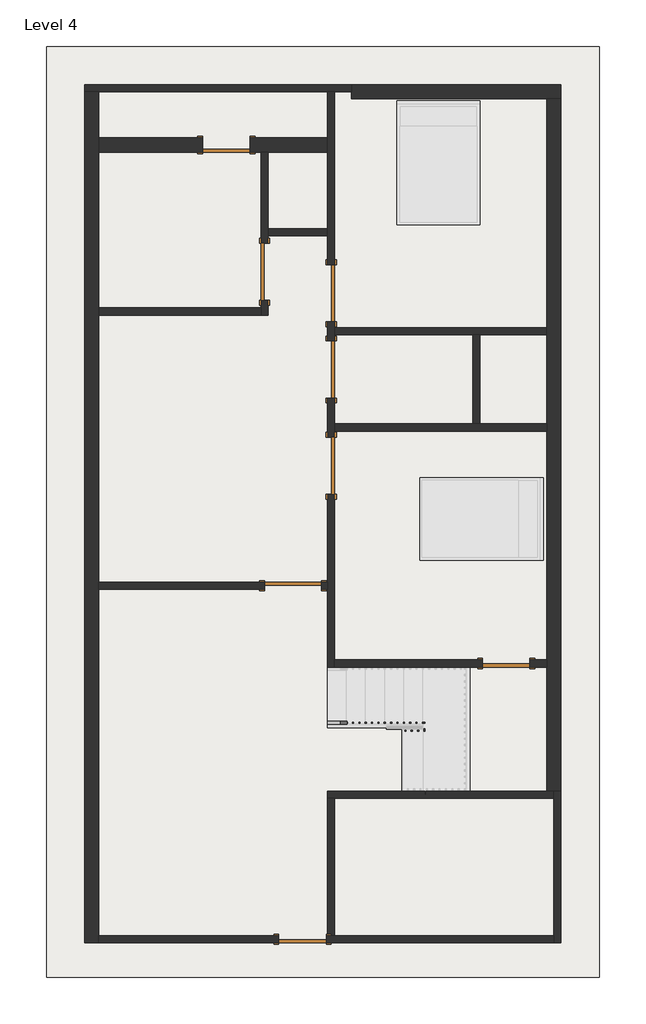
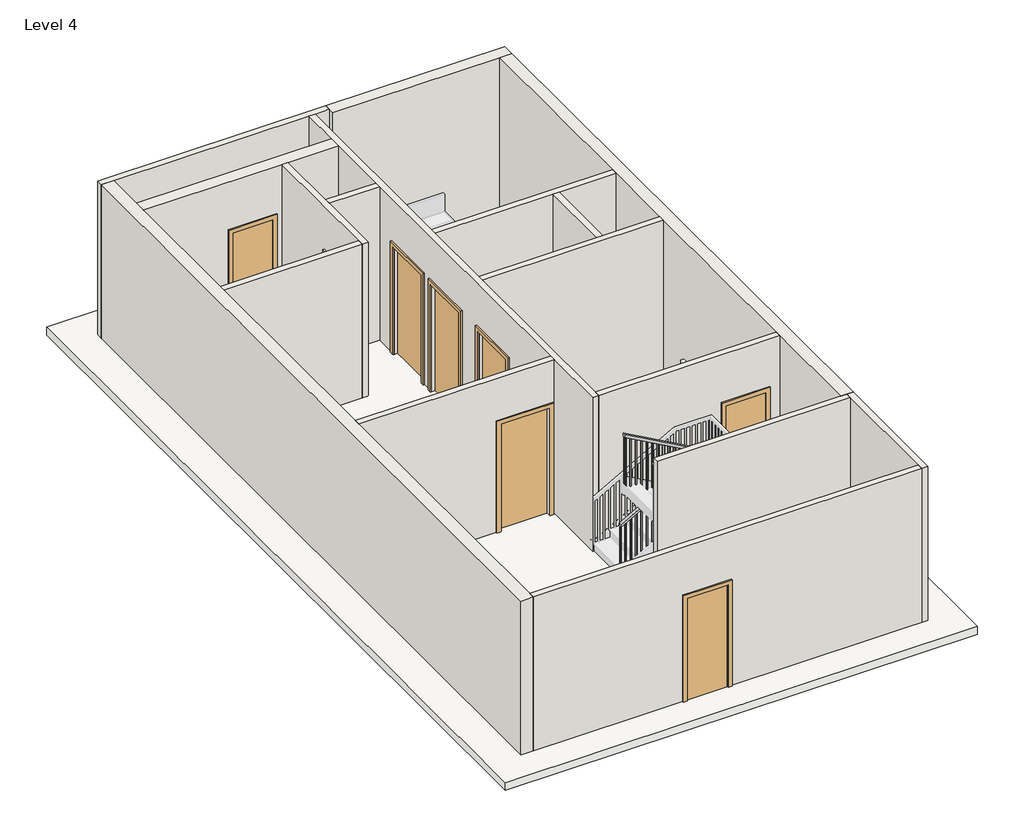
# One storey, part 1 of 2: 18 walls, 8 doors, 1 railing, 1 roof.
"""IFC4 building model written with IfcOpenShell, lengths in millimetres."""

from ifc_helpers import new_model, si_unit, frame, origin, place, context, project, spatial, polyline, outline, extrude, faceted_brep, transform, mapped, element, save
from components import door_85036156, door_d8f5dbb5, door_305aa2a5, door_e5f9f3c4

model = new_model("IFC4")

# Units and contexts
model_context = context("Model", 3, world=origin())
ifc_project = project(units=[si_unit("LENGTHUNIT", "METRE", prefix="MILLI")], contexts=[model_context])

# Site, building, storey
site = spatial("IfcSite", under=ifc_project)
building = spatial("IfcBuilding", under=site)
storey = spatial("IfcBuildingStorey", under=building, Name="Level 4", Elevation=6400.8)

# Doors
placement = place(None, origin())
door_shape = door_85036156(model_context)
element("IfcDoor", 1, ObjectType="Single-Flush : 30\" x 80\"", at=placement, inside=storey, context=model_context, shape_type="MappedRepresentation", body=[
    mapped(door_shape, transform((-2798.2915084, 6430.9935985, 6400.8), x_axis=(1.0, 0.0, 0.0), y_axis=(0.0, 1.0, 0.0), z_axis=(0.0, 0.0, 1.0))),
])
door_2_shape = door_d8f5dbb5(model_context)
element("IfcDoor", 2, ObjectType="Single-Flush : 30\" x 80\"", at=placement, inside=storey, context=model_context, shape_type="MappedRepresentation", body=[
    mapped(door_2_shape, transform((1678.4584916, -1855.7564015, 6400.8), x_axis=(-1.0, 0.0, 0.0), y_axis=(0.0, -1.0, 0.0), z_axis=(0.0, 0.0, 1.0))),
])
element("IfcDoor", 3, ObjectType="Single-Flush : 30\" x 80\"", at=placement, inside=storey, context=model_context, shape_type="MappedRepresentation", body=[
    mapped(door_2_shape, transform((-1579.0915084, -6262.6564015, 6400.8), x_axis=(-1.0, 0.0, 0.0), y_axis=(0.0, -1.0, 0.0), z_axis=(0.0, 0.0, 1.0))),
])
door_3_shape = door_305aa2a5(model_context)
element("IfcDoor", 4, ObjectType="Single-Flush : 36\" x 84\"", at=placement, inside=storey, context=model_context, shape_type="MappedRepresentation", body=[
    mapped(door_3_shape, transform((-2188.6915084, 4405.3435985, 6400.8), x_axis=(0.0, -1.0, 0.0), y_axis=(1.0, 0.0, 0.0), z_axis=(0.0, 0.0, 1.0))),
])
element("IfcDoor", 5, ObjectType="Single-Flush : 36\" x 84\"", at=placement, inside=storey, context=model_context, shape_type="MappedRepresentation", body=[
    mapped(door_3_shape, transform((-1121.8915084, 1306.5435985, 6400.8), x_axis=(0.0, 1.0, 0.0), y_axis=(-1.0, 0.0, 0.0), z_axis=(0.0, 0.0, 1.0))),
])
door_4_shape = door_e5f9f3c4(model_context)
element("IfcDoor", 6, ObjectType="Single-Flush : 36\" x 84\"", at=placement, inside=storey, context=model_context, shape_type="MappedRepresentation", body=[
    mapped(door_4_shape, transform((-1121.8915084, 4062.4435985, 6400.8), x_axis=(0.0, -1.0, 0.0), y_axis=(1.0, 0.0, 0.0), z_axis=(0.0, 0.0, 1.0))),
])
element("IfcDoor", 7, ObjectType="Single-Flush : 36\" x 84\"", at=placement, inside=storey, context=model_context, shape_type="MappedRepresentation", body=[
    mapped(door_4_shape, transform((-1121.8915084, 2843.2435985, 6400.8), x_axis=(0.0, -1.0, 0.0), y_axis=(1.0, 0.0, 0.0), z_axis=(0.0, 0.0, 1.0))),
])
element("IfcDoor", 8, ObjectType="Single-Flush : 36\" x 84\"", at=placement, inside=storey, context=model_context, shape_type="MappedRepresentation", body=[
    mapped(door_4_shape, transform((-1731.4915084, -611.1564015, 6400.8), x_axis=(1.0, 0.0, 0.0), y_axis=(0.0, 1.0, 0.0), z_axis=(0.0, 0.0, 1.0))),
])

# Railing
element("IfcRailing", 9, ObjectType="Handrail - Rectangular", at=placement, inside=storey, context=model_context, shape_type="SolidModel", body=[
    faceted_brep([(-1179.0415084, -2776.5064015, 7484.5333333), (-1179.0415084, -2776.5064015, 7426.420221), (-1179.0415084, -2827.3064015, 7426.420221), (-1179.0415084, -2827.3064015, 7484.5333333), (268.7584916, -2776.5064015, 8288.8666667), (319.5584916, -2776.5064015, 8258.9757765), (319.5584916, -2827.3064015, 8258.9757765), (268.7584916, -2827.3064015, 8288.8666667), (268.7584916, -2776.5064015, 8331.2), (319.5584916, -2776.5064015, 8280.4), (319.5584916, -2827.3064015, 8280.4), (268.7584916, -2827.3064015, 8331.2), (395.7584916, -2776.5064015, 8331.2), (395.7584916, -2776.5064015, 8280.4), (344.9584916, -2827.3064015, 8280.4), (344.9584916, -2827.3064015, 8331.2), (395.7584916, -2903.5064015, 8331.2), (395.7584916, -2903.5064015, 8280.4), (344.9584916, -2903.5064015, 8280.4), (344.9584916, -2903.5064015, 8331.2), (395.7584916, -2928.9064015, 8331.2), (344.9584916, -2928.9064015, 8331.2), (344.9584916, -2928.9064015, 8280.4), (395.7584916, -2928.9064015, 8280.4)], [[[0, 1, 2, 3]], [[1, 0, 4, 5]], [[2, 1, 5, 6]], [[3, 2, 6, 7]], [[0, 3, 7, 4]], [[5, 4, 8, 9]], [[6, 5, 9, 10]], [[7, 6, 10, 11]], [[4, 7, 11, 8]], [[9, 8, 12, 13]], [[10, 9, 13, 14]], [[11, 10, 14, 15]], [[8, 11, 15, 12]], [[13, 12, 16, 17]], [[14, 13, 17, 18]], [[15, 14, 18, 19]], [[12, 15, 19, 16]], [[20, 21, 22, 23]], [[17, 16, 20, 23]], [[18, 17, 23, 22]], [[19, 18, 22, 21]], [[16, 19, 21, 20]]]),
    faceted_brep([(395.7584916, -2903.5064015, 8331.2), (395.7584916, -2954.3064015, 8280.4), (344.9584916, -2954.3064015, 8280.4), (344.9584916, -2903.5064015, 8331.2), (395.7584916, -2903.5064015, 8472.3111111), (344.9584916, -2903.5064015, 8442.420221), (344.9584916, -2954.3064015, 8442.420221), (395.7584916, -2954.3064015, 8472.3111111)], [[[0, 1, 2, 3]], [[4, 5, 6, 7]], [[1, 0, 4, 7]], [[2, 1, 7, 6]], [[3, 2, 6, 5]], [[0, 3, 5, 4]]]),
    faceted_brep([(395.7584916, -2954.3064015, 8472.3111111), (344.9584916, -2954.3064015, 8442.420221), (344.9584916, -2903.5064015, 8442.420221), (395.7584916, -2903.5064015, 8472.3111111), (-1179.0415084, -2954.3064015, 9347.2), (-1179.0415084, -2903.5064015, 9347.2), (-1179.0415084, -2903.5064015, 9289.0868876), (-1179.0415084, -2954.3064015, 9289.0868876)], [[[0, 1, 2, 3]], [[4, 5, 6, 7]], [[1, 0, 4, 7]], [[2, 1, 7, 6]], [[3, 2, 6, 5]], [[0, 3, 5, 4]]]),
    extrude(outline(polyline([(9269.6841099, -1144.1165084), (9280.2674432, -1163.1665084), (8263.4666667, -1163.1665084), (8263.4666667, -1144.1165084), (9269.6841099, -1144.1165084)])), frame((0.0, -2938.4314015, 0.0), z_axis=(0.0, 1.0, 0.0), x_axis=(0.0, 0.0, 1.0)), (0.0, 0.0, 1.0), 19.05),
    extrude(outline(polyline([(9213.2396654, -1042.5165084), (9223.8229988, -1061.5665084), (8263.4666667, -1061.5665084), (8263.4666667, -1042.5165084), (9213.2396654, -1042.5165084)])), frame((0.0, -2938.4314015, 0.0), z_axis=(0.0, 1.0, 0.0), x_axis=(0.0, 0.0, 1.0)), (0.0, 0.0, 1.0), 19.05),
    extrude(outline(polyline([(9156.795221, -940.9165084), (9167.3785543, -959.9665084), (8263.4666667, -959.9665084), (8263.4666667, -940.9165084), (9156.795221, -940.9165084)])), frame((0.0, -2938.4314015, 0.0), z_axis=(0.0, 1.0, 0.0), x_axis=(0.0, 0.0, 1.0)), (0.0, 0.0, 1.0), 19.05),
    extrude(outline(polyline([(9100.3507765, -839.3165084), (9110.9341099, -858.3665084), (8094.1333333, -858.3665084), (8094.1333333, -839.3165084), (9100.3507765, -839.3165084)])), frame((0.0, -2938.4314015, 0.0), z_axis=(0.0, 1.0, 0.0), x_axis=(0.0, 0.0, 1.0)), (0.0, 0.0, 1.0), 19.05),
    extrude(outline(polyline([(9043.9063321, -737.7165084), (9054.4896654, -756.7665084), (8094.1333333, -756.7665084), (8094.1333333, -737.7165084), (9043.9063321, -737.7165084)])), frame((0.0, -2938.4314015, 0.0), z_axis=(0.0, 1.0, 0.0), x_axis=(0.0, 0.0, 1.0)), (0.0, 0.0, 1.0), 19.05),
    extrude(outline(polyline([(8987.4618876, -636.1165084), (8998.045221, -655.1665084), (8094.1333333, -655.1665084), (8094.1333333, -636.1165084), (8987.4618876, -636.1165084)])), frame((0.0, -2938.4314015, 0.0), z_axis=(0.0, 1.0, 0.0), x_axis=(0.0, 0.0, 1.0)), (0.0, 0.0, 1.0), 19.05),
    extrude(outline(polyline([(8931.0174432, -534.5165084), (8941.6007765, -553.5665084), (7924.8, -553.5665084), (7924.8, -534.5165084), (8931.0174432, -534.5165084)])), frame((0.0, -2938.4314015, 0.0), z_axis=(0.0, 1.0, 0.0), x_axis=(0.0, 0.0, 1.0)), (0.0, 0.0, 1.0), 19.05),
    extrude(outline(polyline([(8874.5729988, -432.9165084), (8885.1563321, -451.9665084), (7924.8, -451.9665084), (7924.8, -432.9165084), (8874.5729988, -432.9165084)])), frame((0.0, -2938.4314015, 0.0), z_axis=(0.0, 1.0, 0.0), x_axis=(0.0, 0.0, 1.0)), (0.0, 0.0, 1.0), 19.05),
    extrude(outline(polyline([(8818.1285543, -331.3165084), (8828.7118876, -350.3665084), (7924.8, -350.3665084), (7924.8, -331.3165084), (8818.1285543, -331.3165084)])), frame((0.0, -2938.4314015, 0.0), z_axis=(0.0, 1.0, 0.0), x_axis=(0.0, 0.0, 1.0)), (0.0, 0.0, 1.0), 19.05),
    extrude(outline(polyline([(8761.6841099, -229.7165084), (8772.2674432, -248.7665084), (7755.4666667, -248.7665084), (7755.4666667, -229.7165084), (8761.6841099, -229.7165084)])), frame((0.0, -2938.4314015, 0.0), z_axis=(0.0, 1.0, 0.0), x_axis=(0.0, 0.0, 1.0)), (0.0, 0.0, 1.0), 19.05),
    extrude(outline(polyline([(8705.2396654, -128.1165084), (8715.8229988, -147.1665084), (7755.4666667, -147.1665084), (7755.4666667, -128.1165084), (8705.2396654, -128.1165084)])), frame((0.0, -2938.4314015, 0.0), z_axis=(0.0, 1.0, 0.0), x_axis=(0.0, 0.0, 1.0)), (0.0, 0.0, 1.0), 19.05),
    extrude(outline(polyline([(8648.795221, -26.5165084), (8659.3785543, -45.5665084), (7755.4666667, -45.5665084), (7755.4666667, -26.5165084), (8648.795221, -26.5165084)])), frame((0.0, -2938.4314015, 0.0), z_axis=(0.0, 1.0, 0.0), x_axis=(0.0, 0.0, 1.0)), (0.0, 0.0, 1.0), 19.05),
    extrude(outline(polyline([(8592.3507765, 75.0834916), (8602.9341099, 56.0334916), (7586.1333333, 56.0334916), (7586.1333333, 75.0834916), (8592.3507765, 75.0834916)])), frame((0.0, -2938.4314015, 0.0), z_axis=(0.0, 1.0, 0.0), x_axis=(0.0, 0.0, 1.0)), (0.0, 0.0, 1.0), 19.05),
    extrude(outline(polyline([(8535.9063321, 176.6834916), (8546.4896654, 157.6334916), (7586.1333333, 157.6334916), (7586.1333333, 176.6834916), (8535.9063321, 176.6834916)])), frame((0.0, -2938.4314015, 0.0), z_axis=(0.0, 1.0, 0.0), x_axis=(0.0, 0.0, 1.0)), (0.0, 0.0, 1.0), 19.05),
    extrude(outline(polyline([(8479.4618876, 278.2834916), (8490.045221, 259.2334916), (7586.1333333, 259.2334916), (7586.1333333, 278.2834916), (8479.4618876, 278.2834916)])), frame((0.0, -2938.4314015, 0.0), z_axis=(0.0, 1.0, 0.0), x_axis=(0.0, 0.0, 1.0)), (0.0, 0.0, 1.0), 19.05),
    extrude(outline(polyline([(360.8334916, -2893.9814015), (379.8834916, -2893.9814015), (379.8834916, -2913.0314015), (360.8334916, -2913.0314015), (360.8334916, -2893.9814015)])), frame((0.0, 0.0, 7416.8), z_axis=(0.0, 0.0, 1.0), x_axis=(1.0, 0.0, 0.0)), (0.0, 0.0, 1.0), 863.6),
    extrude(outline(polyline([(335.4334916, -2811.4314015), (335.4334916, -2792.3814015), (354.4834916, -2792.3814015), (354.4834916, -2811.4314015), (335.4334916, -2811.4314015)])), frame((0.0, 0.0, 7416.8), z_axis=(0.0, 0.0, 1.0), x_axis=(1.0, 0.0, 0.0)), (0.0, 0.0, 1.0), 863.6),
    extrude(outline(polyline([(8221.9341099, 252.8834916), (8211.3507765, 233.8334916), (7247.4666667, 233.8334916), (7247.4666667, 252.8834916), (8221.9341099, 252.8834916)])), frame((0.0, -2811.4314015, 0.0), z_axis=(0.0, 1.0, 0.0), x_axis=(0.0, 0.0, 1.0)), (0.0, 0.0, 1.0), 19.05),
    extrude(outline(polyline([(8165.4896654, 151.2834916), (8154.9063321, 132.2334916), (7247.4666667, 132.2334916), (7247.4666667, 151.2834916), (8165.4896654, 151.2834916)])), frame((0.0, -2811.4314015, 0.0), z_axis=(0.0, 1.0, 0.0), x_axis=(0.0, 0.0, 1.0)), (0.0, 0.0, 1.0), 19.05),
    extrude(outline(polyline([(8109.045221, 49.6834916), (8098.4618876, 30.6334916), (7247.4666667, 30.6334916), (7247.4666667, 49.6834916), (8109.045221, 49.6834916)])), frame((0.0, -2811.4314015, 0.0), z_axis=(0.0, 1.0, 0.0), x_axis=(0.0, 0.0, 1.0)), (0.0, 0.0, 1.0), 19.05),
    extrude(outline(polyline([(8052.6007765, -51.9165084), (8042.0174432, -70.9665084), (7078.1333333, -70.9665084), (7078.1333333, -51.9165084), (8052.6007765, -51.9165084)])), frame((0.0, -2811.4314015, 0.0), z_axis=(0.0, 1.0, 0.0), x_axis=(0.0, 0.0, 1.0)), (0.0, 0.0, 1.0), 19.05),
    extrude(outline(polyline([(7996.1563321, -153.5165084), (7985.5729988, -172.5665084), (7078.1333333, -172.5665084), (7078.1333333, -153.5165084), (7996.1563321, -153.5165084)])), frame((0.0, -2811.4314015, 0.0), z_axis=(0.0, 1.0, 0.0), x_axis=(0.0, 0.0, 1.0)), (0.0, 0.0, 1.0), 19.05),
    extrude(outline(polyline([(7939.7118876, -255.1165084), (7929.1285543, -274.1665084), (7078.1333333, -274.1665084), (7078.1333333, -255.1165084), (7939.7118876, -255.1165084)])), frame((0.0, -2811.4314015, 0.0), z_axis=(0.0, 1.0, 0.0), x_axis=(0.0, 0.0, 1.0)), (0.0, 0.0, 1.0), 19.05),
    extrude(outline(polyline([(7883.2674432, -356.7165084), (7872.6841099, -375.7665084), (6908.8, -375.7665084), (6908.8, -356.7165084), (7883.2674432, -356.7165084)])), frame((0.0, -2811.4314015, 0.0), z_axis=(0.0, 1.0, 0.0), x_axis=(0.0, 0.0, 1.0)), (0.0, 0.0, 1.0), 19.05),
    extrude(outline(polyline([(7826.8229988, -458.3165084), (7816.2396654, -477.3665084), (6908.8, -477.3665084), (6908.8, -458.3165084), (7826.8229988, -458.3165084)])), frame((0.0, -2811.4314015, 0.0), z_axis=(0.0, 1.0, 0.0), x_axis=(0.0, 0.0, 1.0)), (0.0, 0.0, 1.0), 19.05),
    extrude(outline(polyline([(7770.3785543, -559.9165084), (7759.795221, -578.9665084), (6908.8, -578.9665084), (6908.8, -559.9165084), (7770.3785543, -559.9165084)])), frame((0.0, -2811.4314015, 0.0), z_axis=(0.0, 1.0, 0.0), x_axis=(0.0, 0.0, 1.0)), (0.0, 0.0, 1.0), 19.05),
    extrude(outline(polyline([(7713.9341099, -661.5165084), (7703.3507765, -680.5665084), (6739.4666667, -680.5665084), (6739.4666667, -661.5165084), (7713.9341099, -661.5165084)])), frame((0.0, -2811.4314015, 0.0), z_axis=(0.0, 1.0, 0.0), x_axis=(0.0, 0.0, 1.0)), (0.0, 0.0, 1.0), 19.05),
    extrude(outline(polyline([(7657.4896654, -763.1165084), (7646.9063321, -782.1665084), (6739.4666667, -782.1665084), (6739.4666667, -763.1165084), (7657.4896654, -763.1165084)])), frame((0.0, -2811.4314015, 0.0), z_axis=(0.0, 1.0, 0.0), x_axis=(0.0, 0.0, 1.0)), (0.0, 0.0, 1.0), 19.05),
    extrude(outline(polyline([(7601.045221, -864.7165084), (7590.4618876, -883.7665084), (6739.4666667, -883.7665084), (6739.4666667, -864.7165084), (7601.045221, -864.7165084)])), frame((0.0, -2811.4314015, 0.0), z_axis=(0.0, 1.0, 0.0), x_axis=(0.0, 0.0, 1.0)), (0.0, 0.0, 1.0), 19.05),
    extrude(outline(polyline([(7544.6007765, -966.3165084), (7534.0174432, -985.3665084), (6570.1333333, -985.3665084), (6570.1333333, -966.3165084), (7544.6007765, -966.3165084)])), frame((0.0, -2811.4314015, 0.0), z_axis=(0.0, 1.0, 0.0), x_axis=(0.0, 0.0, 1.0)), (0.0, 0.0, 1.0), 19.05),
    extrude(outline(polyline([(7488.1563321, -1067.9165084), (7477.5729988, -1086.9665084), (6570.1333333, -1086.9665084), (6570.1333333, -1067.9165084), (7488.1563321, -1067.9165084)])), frame((0.0, -2811.4314015, 0.0), z_axis=(0.0, 1.0, 0.0), x_axis=(0.0, 0.0, 1.0)), (0.0, 0.0, 1.0), 19.05),
    extrude(outline(polyline([(360.8334916, -2919.3814015), (379.8834916, -2919.3814015), (379.8834916, -2938.4314015), (360.8334916, -2938.4314015), (360.8334916, -2919.3814015)])), frame((0.0, 0.0, 7416.8), z_axis=(0.0, 0.0, 1.0), x_axis=(1.0, 0.0, 0.0)), (0.0, 0.0, 1.0), 863.6),
    extrude(outline(polyline([(360.8334916, -2811.4314015), (360.8334916, -2792.3814015), (379.8834916, -2792.3814015), (379.8834916, -2811.4314015), (360.8334916, -2811.4314015)])), frame((0.0, 0.0, 7416.8), z_axis=(0.0, 0.0, 1.0), x_axis=(1.0, 0.0, 0.0)), (0.0, 0.0, 1.0), 863.6),
    extrude(outline(polyline([(9278.5035543, -1159.9915084), (9289.0868876, -1179.0415084), (8263.4666667, -1179.0415084), (8263.4666667, -1159.9915084), (9278.5035543, -1159.9915084)])), frame((0.0, -2938.4314015, 0.0), z_axis=(0.0, 1.0, 0.0), x_axis=(0.0, 0.0, 1.0)), (0.0, 0.0, 1.0), 19.05),
    extrude(outline(polyline([(7437.0035543, -1159.9915084), (7426.420221, -1179.0415084), (6570.1333333, -1179.0415084), (6570.1333333, -1159.9915084), (7437.0035543, -1159.9915084)])), frame((0.0, -2811.4314015, 0.0), z_axis=(0.0, 1.0, 0.0), x_axis=(0.0, 0.0, 1.0)), (0.0, 0.0, 1.0), 19.05),
])

# Roof
element("IfcRoof", 10, ObjectType="Generic - 12\"", at=placement, inside=storey, context=model_context, shape_type="SweptSolid", body=[
    extrude(outline(polyline([(-5674.8415084, 8005.7935985), (3164.3584916, 8005.7935985), (3164.3584916, -6872.2564015), (-5674.8415084, -6872.2564015), (-5674.8415084, 8005.7935985)])), frame((0.0, 0.0, 6248.4), z_axis=(0.0, 0.0, 1.0), x_axis=(1.0, 0.0, 0.0)), (0.0, 0.0, 1.0), 152.4),
])

# Walls
element("IfcWall", 11, ObjectType="WALL 9\"", at=placement, inside=storey, context=model_context, shape_type="Brep", body=[
    faceted_brep([(-798.0415084, 7167.5935985, 6400.8), (2326.1584916, 7167.5935985, 6400.8), (2554.7584916, 7167.5935985, 6400.8), (2554.7584916, 7167.5935985, 9448.8), (2326.1584916, 7167.5935985, 9448.8), (-798.0415084, 7167.5935985, 9448.8), (-798.0415084, 7396.1935985, 6400.8), (-798.0415084, 7396.1935985, 9448.8), (2554.7584916, 7396.1935985, 9448.8), (2554.7584916, 7396.1935985, 6400.8), (-798.0415084, 7281.8935985, 6400.8), (-798.0415084, 7281.8935985, 9448.8)], [[[0, 1, 2, 3, 4, 5]], [[6, 7, 8, 9]], [[2, 1, 0, 10, 6, 9]], [[5, 4, 3, 8, 7, 11]], [[0, 5, 11, 7, 6, 10]], [[3, 2, 9, 8]]]),
])
element("IfcWall", 12, ObjectType="WALL 9\"", at=placement, inside=storey, context=model_context, shape_type="Brep", body=[
    faceted_brep([(2326.1584916, 7167.5935985, 6400.8), (2326.1584916, 3509.9935985, 6400.8), (2326.1584916, 3395.6935985, 6400.8), (2326.1584916, 1973.2935985, 6400.8), (2326.1584916, 1858.9935985, 6400.8), (2326.1584916, -1798.6064015, 6400.8), (2326.1584916, -1912.9064015, 6400.8), (2326.1584916, -3894.1064015, 6400.8), (2326.1584916, -3894.1064015, 9448.8), (2326.1584916, -1912.9064015, 9448.8), (2326.1584916, -1798.6064015, 9448.8), (2326.1584916, 1858.9935985, 9448.8), (2326.1584916, 1973.2935985, 9448.8), (2326.1584916, 3395.6935985, 9448.8), (2326.1584916, 3509.9935985, 9448.8), (2326.1584916, 7167.5935985, 9448.8), (2554.7584916, 7167.5935985, 6400.8), (2554.7584916, 7167.5935985, 9448.8), (2554.7584916, -3894.1064015, 9448.8), (2554.7584916, -3894.1064015, 6400.8), (2440.4584916, -3894.1064015, 6400.8), (2440.4584916, -3894.1064015, 9448.8)], [[[0, 1, 2, 3, 4, 5, 6, 7, 8, 9, 10, 11, 12, 13, 14, 15]], [[16, 17, 18, 19]], [[7, 6, 5, 4, 3, 2, 1, 0, 16, 19, 20]], [[15, 14, 13, 12, 11, 10, 9, 8, 21, 18, 17]], [[0, 15, 17, 16]], [[8, 7, 20, 19, 18, 21]]]),
])
element("IfcWall", 13, ObjectType="WALL 9\"", at=placement, inside=storey, context=model_context, shape_type="Brep", body=[
    faceted_brep([(-5065.2415084, 7281.8935985, 6400.8), (-5065.2415084, -6319.8064015, 6400.8), (-5065.2415084, -6319.8064015, 9448.8), (-5065.2415084, 7281.8935985, 9448.8), (-4836.6415084, 7281.8935985, 6400.8), (-4836.6415084, 7281.8935985, 9448.8), (-4836.6415084, 6545.2935985, 9448.8), (-4836.6415084, 6316.6935985, 9448.8), (-4836.6415084, 3827.4935985, 9448.8), (-4836.6415084, 3713.1935985, 9448.8), (-4836.6415084, -554.0064015, 9448.8), (-4836.6415084, -668.3064015, 9448.8), (-4836.6415084, -6205.5064015, 9448.8), (-4836.6415084, -6319.8064015, 9448.8), (-4836.6415084, -6319.8064015, 6400.8), (-4836.6415084, -6205.5064015, 6400.8), (-4836.6415084, -668.3064015, 6400.8), (-4836.6415084, -554.0064015, 6400.8), (-4836.6415084, 3713.1935985, 6400.8), (-4836.6415084, 3827.4935985, 6400.8), (-4836.6415084, 6316.6935985, 6400.8), (-4836.6415084, 6545.2935985, 6400.8)], [[[0, 1, 2, 3]], [[4, 5, 6, 7, 8, 9, 10, 11, 12, 13, 14, 15, 16, 17, 18, 19, 20, 21]], [[1, 0, 4, 21, 20, 19, 18, 17, 16, 15, 14]], [[3, 2, 13, 12, 11, 10, 9, 8, 7, 6, 5]], [[0, 3, 5, 4]], [[2, 1, 14, 13]]]),
])
element("IfcWall", 14, ObjectType="WALL 9\"", at=placement, inside=storey, context=model_context, shape_type="Brep", body=[
    faceted_brep([(-2417.2915084, 6316.6935985, 8432.8), (-2417.2915084, 6316.6935985, 6400.8), (-2245.8415084, 6316.6935985, 6400.8), (-2131.5415084, 6316.6935985, 6400.8), (-1179.0415084, 6316.6935985, 6400.8), (-1179.0415084, 6316.6935985, 9448.8), (-2131.5415084, 6316.6935985, 9448.8), (-2245.8415084, 6316.6935985, 9448.8), (-4836.6415084, 6316.6935985, 9448.8), (-4836.6415084, 6316.6935985, 6400.8), (-3179.2915084, 6316.6935985, 6400.8), (-3179.2915084, 6316.6935985, 8432.8), (-1179.0415084, 6545.2935985, 6400.8), (-2417.2915084, 6545.2935985, 6400.8), (-2417.2915084, 6545.2935985, 8432.8), (-3179.2915084, 6545.2935985, 8432.8), (-3179.2915084, 6545.2935985, 6400.8), (-4836.6415084, 6545.2935985, 6400.8), (-4836.6415084, 6545.2935985, 9448.8), (-1179.0415084, 6545.2935985, 9448.8)], [[[0, 1, 2, 3, 4, 5, 6, 7, 8, 9, 10, 11]], [[12, 13, 14, 15, 16, 17, 18, 19]], [[10, 9, 17, 16]], [[4, 3, 2, 1, 13, 12]], [[8, 7, 6, 5, 19, 18]], [[9, 8, 18, 17]], [[5, 4, 12, 19]], [[14, 13, 1, 0]], [[15, 14, 0, 11]], [[16, 15, 11, 10]]]),
])
element("IfcWall", 15, ObjectType="WALL4.5\"", at=placement, inside=storey, context=model_context, shape_type="Brep", body=[
    faceted_brep([(-5065.2415084, 7281.8935985, 6400.8), (-4836.6415084, 7281.8935985, 6400.8), (-1179.0415084, 7281.8935985, 6400.8), (-1064.7415084, 7281.8935985, 6400.8), (-798.0415084, 7281.8935985, 6400.8), (-798.0415084, 7281.8935985, 9448.8), (-1064.7415084, 7281.8935985, 9448.8), (-1179.0415084, 7281.8935985, 9448.8), (-4836.6415084, 7281.8935985, 9448.8), (-5065.2415084, 7281.8935985, 9448.8), (-5065.2415084, 7396.1935985, 6400.8), (-5065.2415084, 7396.1935985, 9448.8), (-798.0415084, 7396.1935985, 9448.8), (-798.0415084, 7396.1935985, 6400.8)], [[[0, 1, 2, 3, 4, 5, 6, 7, 8, 9]], [[10, 11, 12, 13]], [[4, 3, 2, 1, 0, 10, 13]], [[5, 4, 13, 12]], [[9, 8, 7, 6, 5, 12, 11]], [[0, 9, 11, 10]]]),
])
element("IfcWall", 16, ObjectType="WALL4.5\"", at=placement, inside=storey, context=model_context, shape_type="Brep", body=[
    faceted_brep([(2554.7584916, -6319.8064015, 6400.8), (2554.7584916, -3894.1064015, 6400.8), (2554.7584916, -3894.1064015, 9448.8), (2554.7584916, -6319.8064015, 9448.8), (2440.4584916, -6319.8064015, 6400.8), (2440.4584916, -6319.8064015, 9448.8), (2440.4584916, -6205.5064015, 9448.8), (2440.4584916, -4008.4064015, 9448.8), (2440.4584916, -3894.1064015, 9448.8), (2440.4584916, -3894.1064015, 6400.8), (2440.4584916, -4008.4064015, 6400.8), (2440.4584916, -6205.5064015, 6400.8)], [[[0, 1, 2, 3]], [[4, 5, 6, 7, 8, 9, 10, 11]], [[1, 0, 4, 11, 10, 9]], [[3, 2, 8, 7, 6, 5]], [[2, 1, 9, 8]], [[0, 3, 5, 4]]]),
])
element("IfcWall", 17, ObjectType="WALL4.5\"", at=placement, inside=storey, context=model_context, shape_type="Brep", body=[
    faceted_brep([(2440.4584916, -3894.1064015, 6400.8), (2326.1584916, -3894.1064015, 6400.8), (-1179.0415084, -3894.1064015, 6400.8), (-1179.0415084, -3894.1064015, 9448.8), (2326.1584916, -3894.1064015, 9448.8), (2440.4584916, -3894.1064015, 9448.8), (2440.4584916, -4008.4064015, 6400.8), (2440.4584916, -4008.4064015, 9448.8), (-1179.0415084, -4008.4064015, 9448.8), (-1179.0415084, -4008.4064015, 7620.0), (-1179.0415084, -4008.4064015, 6400.8), (-1064.7415084, -4008.4064015, 6400.8)], [[[0, 1, 2, 3, 4, 5]], [[6, 7, 8, 9, 10, 11]], [[2, 1, 0, 6, 11, 10]], [[5, 4, 3, 8, 7]], [[0, 5, 7, 6]], [[3, 2, 10, 9, 8]]]),
])
element("IfcWall", 18, ObjectType="WALL4.5\"", at=placement, inside=storey, context=model_context, shape_type="Brep", body=[
    faceted_brep([(-2245.8415084, 3948.1435985, 8534.4), (-2245.8415084, 3948.1435985, 6400.8), (-2245.8415084, 3827.4935985, 6400.8), (-2245.8415084, 3713.1935985, 6400.8), (-2245.8415084, 3713.1935985, 9448.8), (-2245.8415084, 3827.4935985, 9448.8), (-2245.8415084, 6316.6935985, 9448.8), (-2245.8415084, 6316.6935985, 6400.8), (-2245.8415084, 4862.5435985, 6400.8), (-2245.8415084, 4862.5435985, 8534.4), (-2131.5415084, 3713.1935985, 6400.8), (-2131.5415084, 3948.1435985, 6400.8), (-2131.5415084, 3948.1435985, 8534.4), (-2131.5415084, 4862.5435985, 8534.4), (-2131.5415084, 4862.5435985, 6400.8), (-2131.5415084, 4983.1935985, 6400.8), (-2131.5415084, 5097.4935985, 6400.8), (-2131.5415084, 6316.6935985, 6400.8), (-2131.5415084, 6316.6935985, 9448.8), (-2131.5415084, 5097.4935985, 9448.8), (-2131.5415084, 4983.1935985, 9448.8), (-2131.5415084, 3713.1935985, 9448.8)], [[[0, 1, 2, 3, 4, 5, 6, 7, 8, 9]], [[10, 11, 12, 13, 14, 15, 16, 17, 18, 19, 20, 21]], [[8, 7, 17, 16, 15, 14]], [[3, 2, 1, 11, 10]], [[6, 5, 4, 21, 20, 19, 18]], [[7, 6, 18, 17]], [[4, 3, 10, 21]], [[12, 11, 1, 0]], [[13, 12, 0, 9]], [[14, 13, 9, 8]]]),
])
element("IfcWall", 19, ObjectType="WALL4.5\"", at=placement, inside=storey, context=model_context, shape_type="SweptSolid", body=[
    extrude(outline(polyline([(-2245.8415084, 3713.1935985), (-4836.6415084, 3713.1935985), (-4836.6415084, 3827.4935985), (-2245.8415084, 3827.4935985), (-2245.8415084, 3713.1935985)])), frame((0.0, 0.0, 6400.8), z_axis=(0.0, 0.0, 1.0), x_axis=(1.0, 0.0, 0.0)), (0.0, 0.0, 1.0), 3048.0),
])
element("IfcWall", 20, ObjectType="WALL4.5\"", at=placement, inside=storey, context=model_context, shape_type="SweptSolid", body=[
    extrude(outline(polyline([(-1179.0415084, 4983.1935985), (-2131.5415084, 4983.1935985), (-2131.5415084, 5097.4935985), (-1179.0415084, 5097.4935985), (-1179.0415084, 4983.1935985)])), frame((0.0, 0.0, 6400.8), z_axis=(0.0, 0.0, 1.0), x_axis=(1.0, 0.0, 0.0)), (0.0, 0.0, 1.0), 3048.0),
])
element("IfcWall", 21, ObjectType="WALL4.5\"", at=placement, inside=storey, context=model_context, shape_type="Brep", body=[
    faceted_brep([(-1179.0415084, 2386.0435985, 6400.8), (-1179.0415084, 1763.7435985, 6400.8), (-1179.0415084, 1763.7435985, 8534.4), (-1179.0415084, 849.3435985, 8534.4), (-1179.0415084, 849.3435985, 6400.8), (-1179.0415084, -554.0064015, 6400.8), (-1179.0415084, -668.3064015, 6400.8), (-1179.0415084, -1912.9064015, 6400.8), (-1179.0415084, -1912.9064015, 9448.8), (-1179.0415084, -668.3064015, 9448.8), (-1179.0415084, -554.0064015, 9448.8), (-1179.0415084, 4983.1935985, 9448.8), (-1179.0415084, 5097.4935985, 9448.8), (-1179.0415084, 6316.6935985, 9448.8), (-1179.0415084, 6545.2935985, 9448.8), (-1179.0415084, 7281.8935985, 9448.8), (-1179.0415084, 7281.8935985, 6400.8), (-1179.0415084, 6545.2935985, 6400.8), (-1179.0415084, 6316.6935985, 6400.8), (-1179.0415084, 5097.4935985, 6400.8), (-1179.0415084, 4983.1935985, 6400.8), (-1179.0415084, 4519.6435985, 6400.8), (-1179.0415084, 4519.6435985, 8534.4), (-1179.0415084, 3605.2435985, 8534.4), (-1179.0415084, 3605.2435985, 6400.8), (-1179.0415084, 3300.4435985, 6400.8), (-1179.0415084, 3300.4435985, 8534.4), (-1179.0415084, 2386.0435985, 8534.4), (-1064.7415084, 1763.7435985, 8534.4), (-1064.7415084, 1763.7435985, 6400.8), (-1064.7415084, 1858.9935985, 6400.8), (-1064.7415084, 1973.2935985, 6400.8), (-1064.7415084, 2386.0435985, 6400.8), (-1064.7415084, 2386.0435985, 8534.4), (-1064.7415084, 3300.4435985, 8534.4), (-1064.7415084, 3300.4435985, 6400.8), (-1064.7415084, 3395.6935985, 6400.8), (-1064.7415084, 3509.9935985, 6400.8), (-1064.7415084, 3605.2435985, 6400.8), (-1064.7415084, 3605.2435985, 8534.4), (-1064.7415084, 4519.6435985, 8534.4), (-1064.7415084, 4519.6435985, 6400.8), (-1064.7415084, 7281.8935985, 6400.8), (-1064.7415084, 7281.8935985, 9448.8), (-1064.7415084, 3509.9935985, 9448.8), (-1064.7415084, 3395.6935985, 9448.8), (-1064.7415084, 1973.2935985, 9448.8), (-1064.7415084, 1858.9935985, 9448.8), (-1064.7415084, -1798.6064015, 9448.8), (-1064.7415084, -1912.9064015, 9448.8), (-1064.7415084, -1912.9064015, 6400.8), (-1064.7415084, -1798.6064015, 6400.8), (-1064.7415084, 849.3435985, 6400.8), (-1064.7415084, 849.3435985, 8534.4)], [[[0, 1, 2, 3, 4, 5, 6, 7, 8, 9, 10, 11, 12, 13, 14, 15, 16, 17, 18, 19, 20, 21, 22, 23, 24, 25, 26, 27]], [[28, 29, 30, 31, 32, 33, 34, 35, 36, 37, 38, 39, 40, 41, 42, 43, 44, 45, 46, 47, 48, 49, 50, 51, 52, 53]], [[21, 20, 19, 18, 17, 16, 42, 41]], [[25, 24, 38, 37, 36, 35]], [[52, 51, 50, 7, 6, 5, 4]], [[32, 31, 30, 29, 1, 0]], [[15, 14, 13, 12, 11, 10, 9, 8, 49, 48, 47, 46, 45, 44, 43]], [[16, 15, 43, 42]], [[8, 7, 50, 49]], [[39, 38, 24, 23]], [[40, 39, 23, 22]], [[41, 40, 22, 21]], [[33, 32, 0, 27]], [[34, 33, 27, 26]], [[35, 34, 26, 25]], [[2, 1, 29, 28]], [[3, 2, 28, 53]], [[4, 3, 53, 52]]]),
])
element("IfcWall", 22, ObjectType="WALL4.5\"", at=placement, inside=storey, context=model_context, shape_type="SweptSolid", body=[
    extrude(outline(polyline([(6400.8, -1064.7415084), (6400.8, 1297.4584916), (8432.8, 1297.4584916), (8432.8, 2059.4584916), (6400.8, 2059.4584916), (6400.8, 2326.1584916), (9448.8, 2326.1584916), (9448.8, -1064.7415084), (6400.8, -1064.7415084)])), frame((0.0, -1912.9064015, 0.0), z_axis=(0.0, 1.0, 0.0), x_axis=(0.0, 0.0, 1.0)), (0.0, 0.0, 1.0), 114.3),
])
element("IfcWall", 23, ObjectType="WALL4.5\"", at=placement, inside=storey, context=model_context, shape_type="Brep", body=[
    faceted_brep([(-1064.7415084, 3395.6935985, 6400.8), (1145.0584916, 3395.6935985, 6400.8), (1259.3584916, 3395.6935985, 6400.8), (2326.1584916, 3395.6935985, 6400.8), (2326.1584916, 3395.6935985, 9448.8), (1259.3584916, 3395.6935985, 9448.8), (1145.0584916, 3395.6935985, 9448.8), (-1064.7415084, 3395.6935985, 9448.8), (-1064.7415084, 3509.9935985, 6400.8), (-1064.7415084, 3509.9935985, 9448.8), (2326.1584916, 3509.9935985, 9448.8), (2326.1584916, 3509.9935985, 6400.8)], [[[0, 1, 2, 3, 4, 5, 6, 7]], [[8, 9, 10, 11]], [[3, 2, 1, 0, 8, 11]], [[7, 6, 5, 4, 10, 9]], [[4, 3, 11, 10]], [[0, 7, 9, 8]]]),
])
element("IfcWall", 24, ObjectType="WALL4.5\"", at=placement, inside=storey, context=model_context, shape_type="SweptSolid", body=[
    extrude(outline(polyline([(1259.3584916, 3395.6935985), (1259.3584916, 1973.2935985), (1145.0584916, 1973.2935985), (1145.0584916, 3395.6935985), (1259.3584916, 3395.6935985)])), frame((0.0, 0.0, 6400.8), z_axis=(0.0, 0.0, 1.0), x_axis=(1.0, 0.0, 0.0)), (0.0, 0.0, 1.0), 3048.0),
])
element("IfcWall", 25, ObjectType="WALL4.5\"", at=placement, inside=storey, context=model_context, shape_type="Brep", body=[
    faceted_brep([(-1064.7415084, 1858.9935985, 6400.8), (2326.1584916, 1858.9935985, 6400.8), (2326.1584916, 1858.9935985, 9448.8), (-1064.7415084, 1858.9935985, 9448.8), (-1064.7415084, 1973.2935985, 6400.8), (-1064.7415084, 1973.2935985, 9448.8), (1145.0584916, 1973.2935985, 9448.8), (1259.3584916, 1973.2935985, 9448.8), (2326.1584916, 1973.2935985, 9448.8), (2326.1584916, 1973.2935985, 6400.8), (1259.3584916, 1973.2935985, 6400.8), (1145.0584916, 1973.2935985, 6400.8)], [[[0, 1, 2, 3]], [[4, 5, 6, 7, 8, 9, 10, 11]], [[1, 0, 4, 11, 10, 9]], [[3, 2, 8, 7, 6, 5]], [[2, 1, 9, 8]], [[0, 3, 5, 4]]]),
])
element("IfcWall", 26, ObjectType="WALL4.5\"", at=placement, inside=storey, context=model_context, shape_type="SweptSolid", body=[
    extrude(outline(polyline([(8534.4, -1274.2915084), (6400.8, -1274.2915084), (6400.8, -1179.0415084), (9448.8, -1179.0415084), (9448.8, -4836.6415084), (6400.8, -4836.6415084), (6400.8, -2188.6915084), (8534.4, -2188.6915084), (8534.4, -1274.2915084)])), frame((0.0, -668.3064015, 0.0), z_axis=(0.0, 1.0, 0.0), x_axis=(0.0, 0.0, 1.0)), (0.0, 0.0, 1.0), 114.3),
])
element("IfcWall", 27, ObjectType="WALL4.5\"", at=placement, inside=storey, context=model_context, shape_type="SweptSolid", body=[
    extrude(outline(polyline([(-1179.0415084, -6205.5064015), (-1179.0415084, -4008.4064015), (-1064.7415084, -4008.4064015), (-1064.7415084, -6205.5064015), (-1179.0415084, -6205.5064015)])), frame((0.0, 0.0, 6400.8), z_axis=(0.0, 0.0, 1.0), x_axis=(1.0, 0.0, 0.0)), (0.0, 0.0, 1.0), 1219.2),
])
element("IfcWall", 28, ObjectType="WALL4.5\"", at=placement, inside=storey, context=model_context, shape_type="Brep", body=[
    faceted_brep([(-4836.6415084, -6319.8064015, 6400.8), (-1960.0915084, -6319.8064015, 6400.8), (-1960.0915084, -6319.8064015, 8432.8), (-1198.0915084, -6319.8064015, 8432.8), (-1198.0915084, -6319.8064015, 6400.8), (2440.4584916, -6319.8064015, 6400.8), (2440.4584916, -6319.8064015, 9448.8), (-4836.6415084, -6319.8064015, 9448.8), (-1960.0915084, -6205.5064015, 8432.8), (-1960.0915084, -6205.5064015, 6400.8), (-4836.6415084, -6205.5064015, 6400.8), (-4836.6415084, -6205.5064015, 9448.8), (2440.4584916, -6205.5064015, 9448.8), (2440.4584916, -6205.5064015, 6400.8), (-1064.7415084, -6205.5064015, 6400.8), (-1179.0415084, -6205.5064015, 6400.8), (-1198.0915084, -6205.5064015, 6400.8), (-1198.0915084, -6205.5064015, 8432.8)], [[[0, 1, 2, 3, 4, 5, 6, 7]], [[8, 9, 10, 11, 12, 13, 14, 15, 16, 17]], [[10, 9, 1, 0]], [[16, 15, 14, 13, 5, 4]], [[7, 6, 12, 11]], [[0, 7, 11, 10]], [[6, 5, 13, 12]], [[2, 1, 9, 8]], [[3, 2, 8, 17]], [[4, 3, 17, 16]]]),
])

save(model, "model.ifc")

# Revit data of these elements
# Type "Single-Flush : 30\" x 80\""
#   Type Mark = "5"
#   Construction Type Id = "MDOOR"
#   Assembly Code = "C1020"
#   Analytic Construction = "Metal"
#   Thickness = 0' - 2"
#   Heat Transfer Coefficient (U) = 0.651978 BTU/(h·ft²·°F)
#   Height = 6' - 8"
#   Trim Projection Ext = 0' - 1"
#   Trim Projection Int = 0' - 1"
#   Trim Width = 0' - 3"
#   Width = 2' - 6"
#   Define Thermal Properties by = 1
#   Define Thermal Properties by = 1
#   Door Material = Door - Panel
#   Frame Material = Door - Frame
#   Visual Light Transmittance = 0
#   Solar Heat Gain Coefficient = 0
#   Function = (empty or 0)
#   Wall Closure = (empty or 0)
# Type "Single-Flush : 36\" x 84\""
#   Type Mark = "1"
#   Construction Type Id = "MDOOR"
#   Assembly Code = "C1020"
#   Analytic Construction = "Metal"
#   Thickness = 0' - 2"
#   Heat Transfer Coefficient (U) = 0.651978 BTU/(h·ft²·°F)
#   Height = 7' - 0"
#   Trim Projection Ext = 0' - 1"
#   Trim Projection Int = 0' - 1"
#   Trim Width = 0' - 3"
#   Width = 3' - 0"
#   Define Thermal Properties by = 1
#   Define Thermal Properties by = 1
#   Door Material = Door - Panel
#   Frame Material = Door - Frame
#   Visual Light Transmittance = 0
#   Solar Heat Gain Coefficient = 0
#   Function = (empty or 0)
#   Wall Closure = (empty or 0)
# Type "Handrail - Rectangular"
#   Assembly Code = "C2010400"
#   built-in parameter 1008612 = 0.0416667 (stored number, unit not read)
#   built-in parameter 1008611 = 0.0416667 (stored number, unit not read)
#   built-in parameter 1008609 = 0.333333 (stored number, unit not read)
#   built-in parameter 1008604 = 0.166667 (stored number, unit not read)
#   built-in parameter 1008603 = 0.166667 (stored number, unit not read)
#   Railing Height = 3' - 0"
#   built-in parameter 1008630 = 2
#   built-in parameter 1008610 = 2
#   built-in parameter 1008618 = Baluster - Square : 3/4"
# Type "Generic - 12\""
#   Assembly Code = "B1020"
#   Layers, outside or top first: 0' - 6" no material (function 1)
# Type "WALL 9\""
#   Assembly Code = "B2010"
#   Layers, outside or top first: 0' - 9" no material (function 1)
# Type "WALL4.5\""
#   Assembly Code = "B2010"
#   Layers, outside or top first: 0' - 4 1/2" no material (function 1)
# Elements 1, 2, 3 (IfcDoor, "Single-Flush : 30\" x 80\"")
#   Phase Created = New Construction
#   Materials on its faces: "Door - Frame", "Door - Panel"
# Elements 4, 5, 6, 7, 8 (IfcDoor, "Single-Flush : 36\" x 84\"")
#   Phase Created = New Construction
#   Materials on its faces: "Door - Frame", "Door - Panel"
# Element 9 (IfcRailing, "Handrail - Rectangular")
#   Phase Created = New Construction
# Element 10 (IfcRoof, "Generic - 12\"")
#   built-in parameter 1001705 = 21 (stored number, unit not read)
#   built-in parameter 1001701 = -0.5 (stored number, unit not read)
#   built-in parameter 1001710 = 33615
#   Phase Created = New Construction
#   Materials on its faces: "Default Roof"
# Elements 11, 12, 13 (IfcWall, "WALL 9\"")
#   Top Offset = 0' - 0"
#   Base Offset = 0' - 0"
#   Unconnected Height = 10' - 0"
#   wall height = 10' - 0"
#   Phase Created = New Construction
#   Base Constraint = Level 4
#   Materials on its faces: "Default Wall", "Brick, Common"
# Element 14 (IfcWall, "WALL 9\"")
#   Top Offset = 0' - 0"
#   Base Offset = 0' - 0"
#   Unconnected Height = 10' - 0"
#   wall height = 10' - 0"
#   Phase Created = New Construction
#   Base Constraint = Level 4
#   Materials on its faces: "Default Wall"
# Elements 15, 16, 28 (IfcWall, "WALL4.5\"")
#   Top Offset = 0' - 0"
#   Base Offset = 0' - 0"
#   Unconnected Height = 10' - 0"
#   wall height = 10' - 0"
#   Phase Created = New Construction
#   Base Constraint = Level 4
#   Materials on its faces: "Default Wall", "Brick, Common"
# Elements 17, 18, 19, 20, 21, 22, 23, 24, 25, 26 (IfcWall, "WALL4.5\"")
#   Top Offset = 0' - 0"
#   Base Offset = 0' - 0"
#   Unconnected Height = 10' - 0"
#   wall height = 10' - 0"
#   Phase Created = New Construction
#   Base Constraint = Level 4
#   Materials on its faces: "Default Wall"
# Element 27 (IfcWall, "WALL4.5\"")
#   Top Offset = 0' - 0"
#   Base Offset = 0' - 0"
#   Unconnected Height = 4' - 0"
#   wall height = 4' - 0"
#   Phase Created = New Construction
#   Base Constraint = Level 4
#   Materials on its faces: "Default Wall"
# Materials
#   "Door - Panel": class "Wood", colour RGB 210 159 95, transparency 0, Cost = 0
#   "Door - Frame": colour RGB 118 70 51, transparency 0, Cost = 0
#   "Default Roof": colour RGB 88 101 114, transparency 0, Cost = 0
#   "Default Wall": colour RGB 128 128 128, transparency 0, Cost = 0
#   "Brick, Common": class "Masonry", colour RGB 170 98 104, transparency 0, Description = "Common brick", Cost = 0
